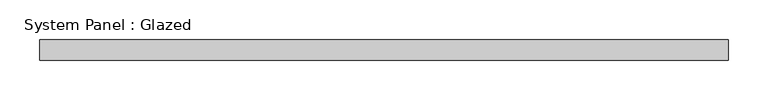
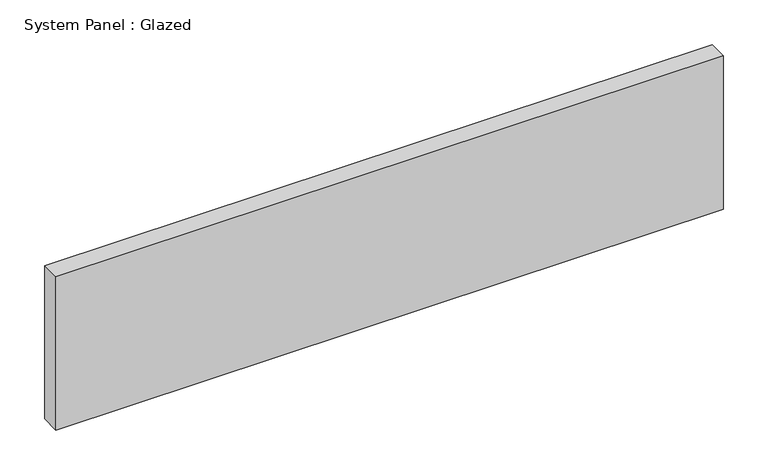
"""IFC4 building model written with IfcOpenShell, lengths in millimetres: plate geometry, System Panel : Glazed."""

from ifc_helpers import new_model, si_unit, origin, origin_with_axes, place, context, project, spatial, polyline, outline, extrude, source, transform, mapped, element, save


def system_panel_glazed_34f1e917(model_context):
    return source(origin(), model_context, "Body", "SweptSolid", [
        extrude(outline(polyline([(431.8, 19.05), (-431.8, 19.05), (-431.8, 44.45), (431.8, 44.45), (431.8, 19.05)])), origin_with_axes(), (0.0, 0.0, 1.0), 209.55),
    ])


if __name__ == "__main__":
    model = new_model("IFC4")
    model_context = context("Model", 3, world=origin())
    ifc_project = project(units=[si_unit("LENGTHUNIT", "METRE", prefix="MILLI")], contexts=[model_context])
    site = spatial("IfcSite", under=ifc_project)
    building = spatial("IfcBuilding", under=site)
    placement = place(None, origin())
    system_panel_glazed_shape = system_panel_glazed_34f1e917(model_context)
    element("IfcPlate", 1, ObjectType="System Panel : Glazed", at=placement, inside=building, context=model_context, shape_type="MappedRepresentation", body=[
        mapped(system_panel_glazed_shape, transform((0.0, 0.0, 0.0), x_axis=(1.0, 0.0, 0.0), y_axis=(0.0, 1.0, 0.0), z_axis=(0.0, 0.0, 1.0))),
    ])
    save(model, "model.ifc")

# Revit data of these elements
# Type "System Panel : Glazed"
#   Construction Type Id = "GSP4R"
#   Analytic Construction = "1/8 in Pilkington single glazing"
#   Visual Light Transmittance = 0.9
#   Solar Heat Gain Coefficient = 0.86
#   Heat Transfer Coefficient (U) = 1.18115 BTU/(h·ft²·°F)
#   Define Thermal Properties by = 1
# Element 1 (IfcPlate, "System Panel : Glazed")
#   Materials on its faces: "Glass"
# Materials
#   "Glass": class "Glass", colour RGB 0 128 192, transparency 0.75, Description = "Soda Lime Glass", Cost = 0
